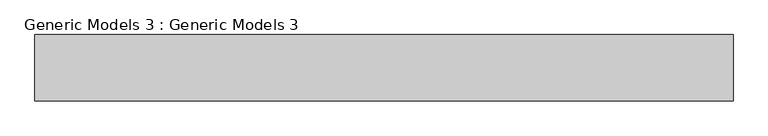
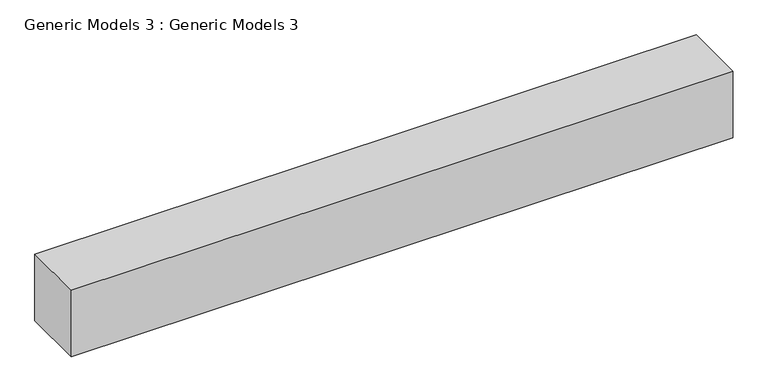
"""IFC4 building model written with IfcOpenShell, lengths in millimetres: proxy geometry, Generic Models 3 : Generic Models 3."""

from ifc_helpers import new_model, si_unit, frame, origin, place, context, project, spatial, polyline, outline, extrude, source, transform, mapped, element, save


def generic_models_3_generic_models_3_43ac32e0(model_context):
    return source(origin(), model_context, "Body", "SweptSolid", [
        extrude(outline(polyline([(25489.814721, -14046.0842441), (6670.0040857, -14046.0842441), (6670.0040857, -12253.1237084), (25489.814721, -12253.1237084), (25489.814721, -14046.0842441)])), frame((0.0, 0.0, 58789.9443989), z_axis=(0.0, 0.0, 1.0), x_axis=(1.0, 0.0, 0.0)), (0.0, 0.0, 1.0), 1997.8223895),
    ])


if __name__ == "__main__":
    model = new_model("IFC4")
    model_context = context("Model", 3, world=origin())
    ifc_project = project(units=[si_unit("LENGTHUNIT", "METRE", prefix="MILLI")], contexts=[model_context])
    site = spatial("IfcSite", under=ifc_project)
    building = spatial("IfcBuilding", under=site)
    placement = place(None, origin())
    generic_models_3_generic_models_3_shape = generic_models_3_generic_models_3_43ac32e0(model_context)
    element("IfcBuildingElementProxy", 1, Name="Generic Models 3 : Generic Models 3", ObjectType="Generic Models 3 : Generic Models 3", at=placement, inside=building, context=model_context, shape_type="MappedRepresentation", body=[
        mapped(generic_models_3_generic_models_3_shape, transform((0.0, 0.0, 0.0), x_axis=(1.0, 0.0, 0.0), y_axis=(0.0, 1.0, 0.0), z_axis=(0.0, 0.0, 1.0))),
    ])
    save(model, "model.ifc")
